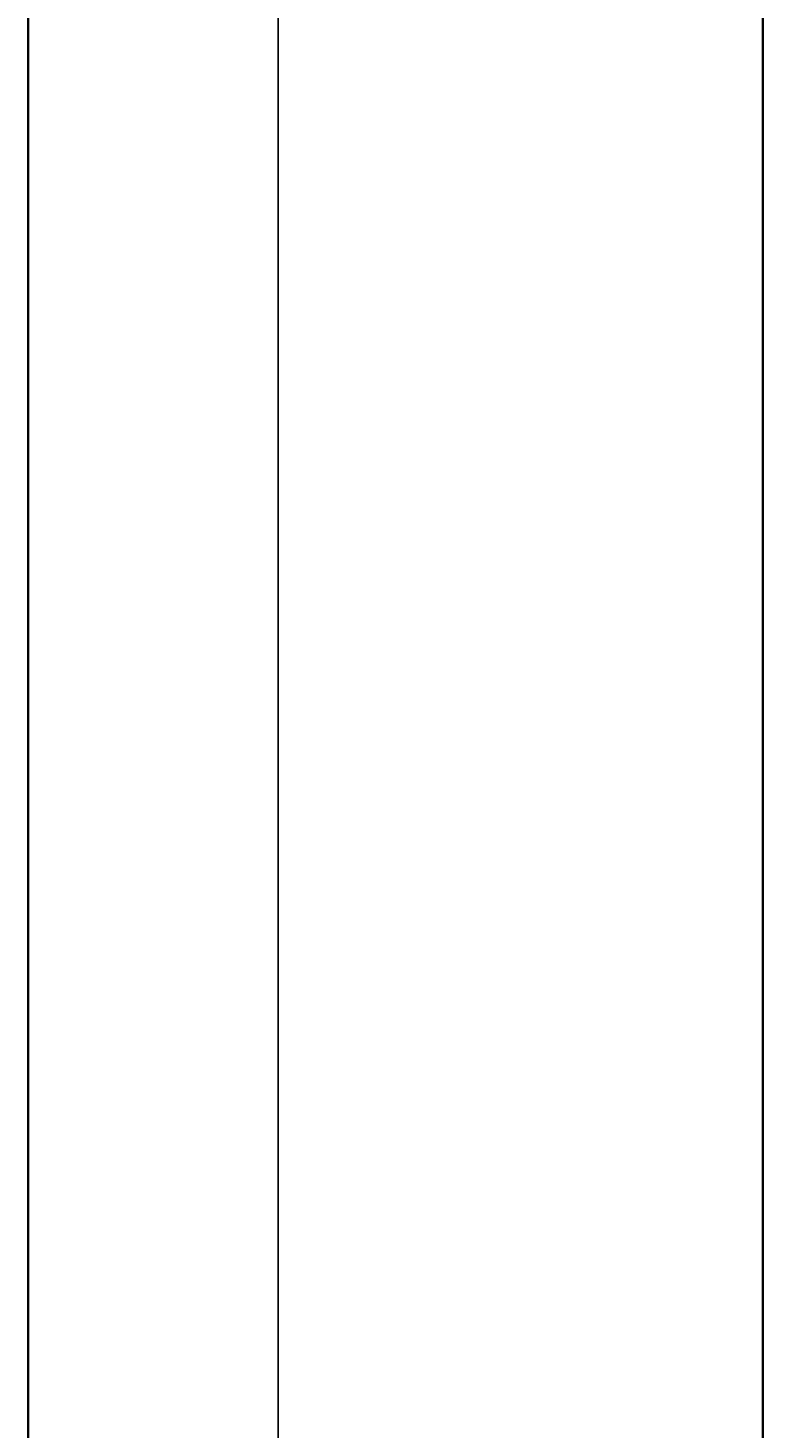
# Model space of a CAD drawing. Units: inches. Extents: x 1088 to 1703, y 668 to 1875.
# Tile 8 of 45: x 1088 to 1173, y 1416 to 1572. Entities that reach past the tile are written whole.
import ezdxf

# ---------------------------------------------------------------- set-up
doc = ezdxf.new("R2010")
doc.units = ezdxf.units.IN
for name, color, linetype, lineweight in [('A-ANNO-DIMS', 2, 'Continuous', 18), ('A-ANNO-TTLB', 7, 'Continuous', 35), ('A-WALL', 7, 'Continuous', 35)]:
    doc.layers.add(name, color=color, linetype=linetype, lineweight=lineweight)
doc.styles.get("Standard").update_dxf_attribs({"font": 'arial.ttf'})
doc.dimstyles.get("Standard").update_dxf_attribs({"dimtxt": 0.18, "dimasz": 0.18, "dimexe": 0.18, "dimexo": 0.0625, "dimgap": 0.09, "dimtad": 0, "dimtih": 1, "dimtoh": 1, "dimdec": 4, "dimzin": 0, "dimdsep": 46, "dimtxsty": 'Standard', "dimcen": 0.09, "dimadec": 0, "dimazin": 0, "dimtfac": 1, "dimtdec": 4, "dimtofl": 0, "dimtmove": 0, "dimatfit": 3, "dimfxl": 1, "dimtolj": 1, "dimtzin": 0, "dimarcsym": 0})

# ---------------------------------------------------------------- blocks, each defined once
blk = doc.blocks.new('*D29')
at = {"layer": 'A-ANNO-DIMS', "color": 0, "lineweight": -2, "transparency": 16777216}
for p, q in [((1170.28, 1803.56), (1116.11, 1803.56)), ((1116.29, 1803.38), (1116.29, 1291.85)), ((1116.29, 779.96), (1116.29, 1291.49)), ((1170.28, 779.78), (1116.11, 779.78))]:
    blk.add_line(p, q, dxfattribs=at)
at = {"layer": 'A-ANNO-DIMS', "color": 0, "transparency": 16777216}
for points in [[(1116.26, 1803.38), (1116.32, 1803.38), (1116.29, 1803.56)], [(1116.26, 779.96), (1116.32, 779.96), (1116.29, 779.78)]]:
    blk.add_solid(points, dxfattribs=at)
at = {"layer": 'Defpoints', "color": 0, "transparency": 16777216}
for p in [(1116.29, 1803.56), (1170.34, 1803.56), (1170.34, 779.78)]:
    blk.add_point(p, dxfattribs=at)
at = {"layer": 'A-ANNO-DIMS', "color": 0, "transparency": 16777216, "insert": (1116.29, 1291.67), "char_height": 0.18, "attachment_point": 5}
blk.add_mtext('\\A1;1023.8', dxfattribs=at)

msp = doc.modelspace()

# ---------------------------------------------------------------- linework, layer by layer
at = {"layer": 'A-ANNO-TTLB'}
msp.add_lwpolyline([(1088.369, 1874.677), (1703.181, 1874.677), (1703.181, 667.947), (1088.369, 667.947)], close=True, dxfattribs=at)
at = {"layer": 'A-WALL'}
msp.add_line((1170.345, 1803.558), (1170.345, 836.058), dxfattribs=at)

# ---------------------------------------------------------------- dimensions: what is measured, and where the dimension line sits
at = {"layer": 'A-ANNO-DIMS'}
dim = msp.add_linear_dim(base=(1116.295, 1803.558), p1=(1170.345, 779.779), p2=(1170.345, 1803.558), angle=90, dimstyle='Standard', override={"dimdec": 1, "dimlfac": 1, "dimrnd": 0, "dimzin": 0, "dimdsep": 46, "dimlunit": 2}, dxfattribs=at)
dim.commit()
dim.dimension.update_dxf_attribs({"geometry": '*D29', "text_midpoint": (1116.295, 1291.669)})

doc.saveas('drawing.dxf')
